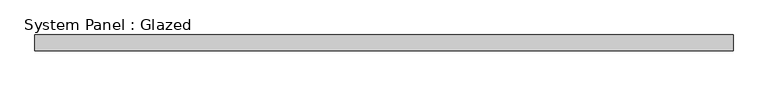
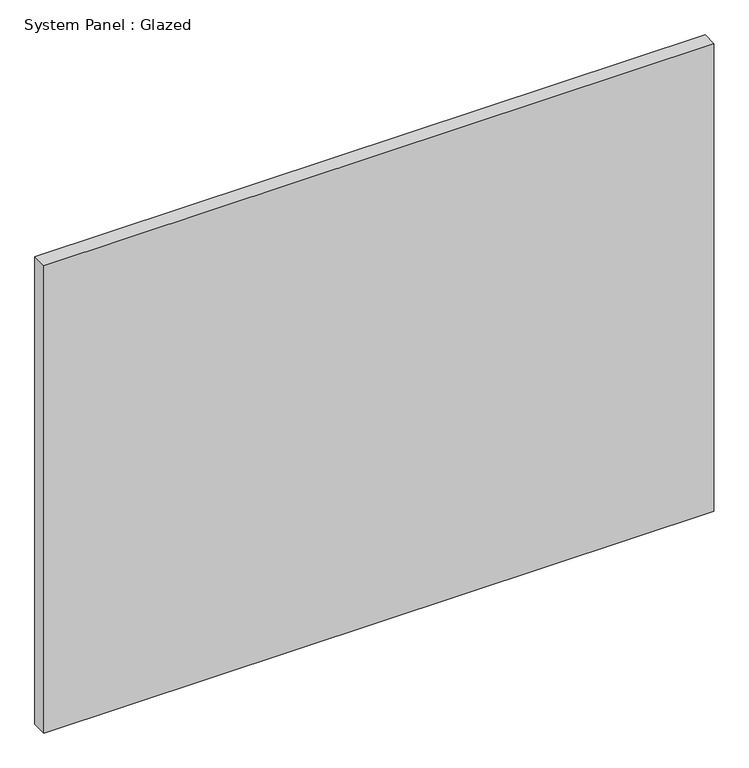
"""IFC4 building model written with IfcOpenShell, lengths in millimetres: plate geometry, System Panel : Glazed."""

from ifc_helpers import new_model, si_unit, origin, origin_with_axes, place, context, project, spatial, polyline, outline, extrude, source, transform, mapped, element, save


def system_panel_glazed_a205a7ab(model_context):
    return source(origin(), model_context, "Body", "SweptSolid", [
        extrude(outline(polyline([(555.3125873, 19.05), (-555.3125873, 19.05), (-555.3125873, 44.45), (555.3125873, 44.45), (555.3125873, 19.05)])), origin_with_axes(), (0.0, 0.0, 1.0), 819.15),
    ])


if __name__ == "__main__":
    model = new_model("IFC4")
    model_context = context("Model", 3, world=origin())
    ifc_project = project(units=[si_unit("LENGTHUNIT", "METRE", prefix="MILLI")], contexts=[model_context])
    site = spatial("IfcSite", under=ifc_project)
    building = spatial("IfcBuilding", under=site)
    placement = place(None, origin())
    system_panel_glazed_shape = system_panel_glazed_a205a7ab(model_context)
    element("IfcPlate", 1, ObjectType="System Panel : Glazed", at=placement, inside=building, context=model_context, shape_type="MappedRepresentation", body=[
        mapped(system_panel_glazed_shape, transform((0.0, 0.0, 0.0), x_axis=(1.0, 0.0, 0.0), y_axis=(0.0, 1.0, 0.0), z_axis=(0.0, 0.0, 1.0))),
    ])
    save(model, "model.ifc")

# Revit data of these elements
# Type "System Panel : Glazed"
#   Construction Type Id = "GSP4R"
#   Analytic Construction = "1/8 in Pilkington single glazing"
#   Visual Light Transmittance = 0.9
#   Solar Heat Gain Coefficient = 0.86
#   Heat Transfer Coefficient (U) = 1.18115 BTU/(h·ft²·°F)
# Element 1 (IfcPlate, "System Panel : Glazed")
#   Materials on its faces: "Glass"
# Materials
#   "Glass": class "Glass", colour RGB 0 128 192, transparency 0.75, Description = "Soda Lime Glass", Cost = 0
